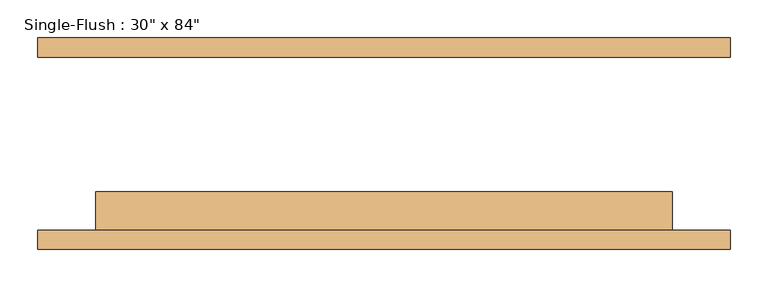
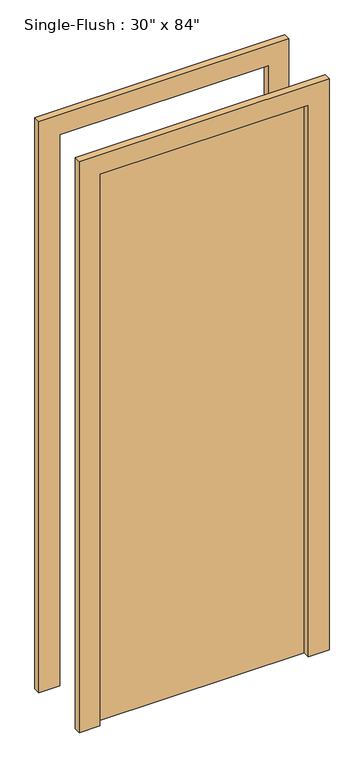
"""IFC4 building model written with IfcOpenShell, lengths in millimetres: door geometry."""

from ifc_helpers import new_model, si_unit, frame, origin, origin_with_axes, place, context, project, spatial, polyline, outline, extrude, source, transform, mapped, element, save


def door_5e1232af(model_context):
    return source(origin(), model_context, "Body", "SweptSolid", [
        extrude(outline(polyline([(2209.8, -457.2), (0.0, -457.2), (0.0, -381.0), (2133.6, -381.0), (2133.6, 381.0), (0.0, 381.0), (0.0, 457.2), (2209.8, 457.2), (2209.8, -457.2)])), frame((0.0, -139.7, 0.0), z_axis=(0.0, 1.0, 0.0), x_axis=(0.0, 0.0, 1.0)), (0.0, 0.0, 1.0), 25.4),
        extrude(outline(polyline([(2209.8, 457.2), (2209.8, -457.2), (0.0, -457.2), (0.0, -381.0), (2133.6, -381.0), (2133.6, 381.0), (0.0, 381.0), (0.0, 457.2), (2209.8, 457.2)])), frame((0.0, 114.3, 0.0), z_axis=(0.0, 1.0, 0.0), x_axis=(0.0, 0.0, 1.0)), (0.0, 0.0, 1.0), 25.4),
        extrude(outline(polyline([(381.0, -63.5), (381.0, -114.3), (-381.0, -114.3), (-381.0, -63.5), (381.0, -63.5)])), origin_with_axes(), (0.0, 0.0, 1.0), 2133.6),
    ])


if __name__ == "__main__":
    model = new_model("IFC4")
    model_context = context("Model", 3, world=origin())
    ifc_project = project(units=[si_unit("LENGTHUNIT", "METRE", prefix="MILLI")], contexts=[model_context])
    site = spatial("IfcSite", under=ifc_project)
    building = spatial("IfcBuilding", under=site)
    placement = place(None, origin())
    door_shape = door_5e1232af(model_context)
    element("IfcDoor", 1, ObjectType="Single-Flush : 30\" x 84\"", at=placement, inside=building, context=model_context, shape_type="MappedRepresentation", body=[
        mapped(door_shape, transform((0.0, 0.0, 0.0), x_axis=(1.0, 0.0, 0.0), y_axis=(0.0, 1.0, 0.0), z_axis=(0.0, 0.0, 1.0))),
    ])
    save(model, "model.ifc")

# Revit data of these elements
# Type "Single-Flush : 30\" x 84\""
#   Type Mark = "4"
#   Assembly Code = "C1020"
#   Thickness = 0' - 2"
#   Height = 7' - 0"
#   Trim Projection Ext = 0' - 1"
#   Trim Projection Int = 0' - 1"
#   Trim Width = 0' - 3"
#   Width = 2' - 6"
#   Door Material = Door - Panel
#   Frame Material = Door - Frame
#   Function = (empty or 0)
#   Wall Closure = (empty or 0)
# Element 1 (IfcDoor, "Single-Flush : 30\" x 84\"")
#   Materials on its faces: "Door - Frame", "Door - Panel"
# Materials
#   "Door - Panel": class "Wood", colour RGB 114 82 51, transparency 0
#   "Door - Frame": colour RGB 153 76 43, transparency 0
